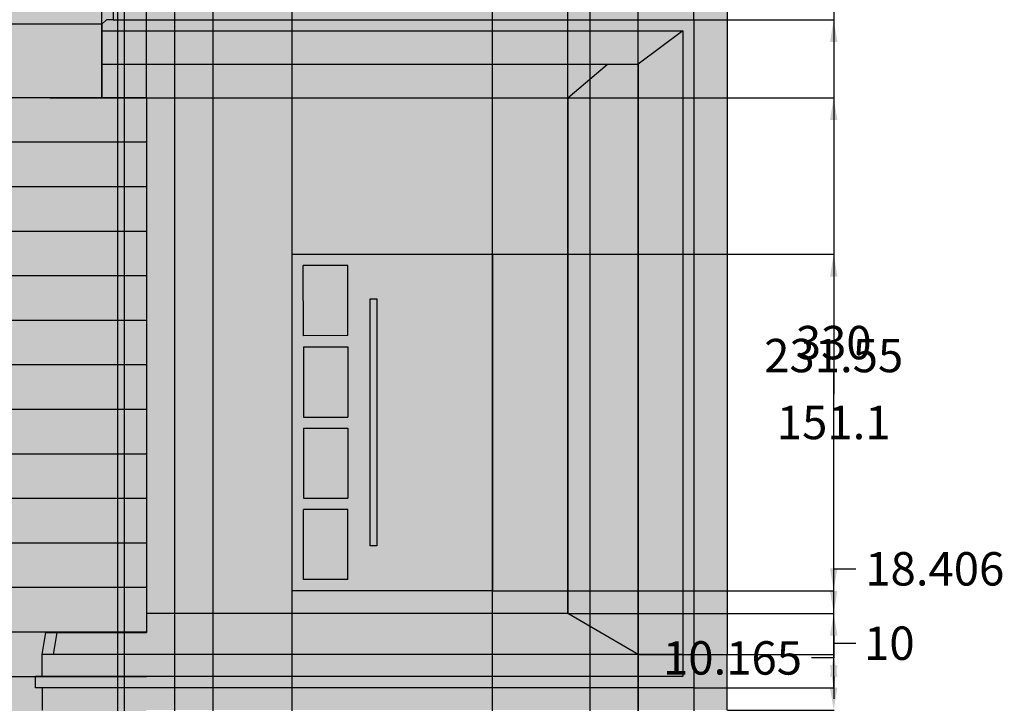
# Model space of a CAD drawing. Units: millimetres. Extents: x 131 to 845, y -20 to 1043.
# Tile 10 of 11: x 403 to 845, y 492 to 799. Entities that reach past the tile are written whole.
import ezdxf

# ---------------------------------------------------------------- set-up
doc = ezdxf.new("R2010")
doc.units = ezdxf.units.MM
doc.header["$MEASUREMENT"] = 0
for name, color, linetype, lineweight in [('A-ANNO-DIMS', 2, 'Continuous', 18), ('A-DOOR', 3, 'Continuous', 25), ('A-DOOR-PATT', 45, 'Continuous', 13), ('A-ELEV', 7, 'Continuous', 25), ('A-ELEV-PATT', 7, 'Continuous', 13), ('A-GLAZ-PATT', 143, 'Continuous', 13), ('A-WALL-PATT', 131, 'Continuous', 13)]:
    doc.layers.add(name, color=color, linetype=linetype, lineweight=lineweight)
doc.styles.get("Standard").update_dxf_attribs({"font": 'arial.ttf'})
doc.dimstyles.get("Standard").update_dxf_attribs({"dimtxt": 15, "dimasz": 10, "dimexe": 0.18, "dimexo": 0.0625, "dimgap": 5, "dimtad": 0, "dimtih": 1, "dimtoh": 1, "dimdec": 0, "dimzin": 0, "dimdsep": 46, "dimtxsty": 'Standard', "dimcen": 5, "dimadec": 0, "dimazin": 0, "dimtfac": 1, "dimtdec": 0, "dimtofl": 0, "dimtmove": 0, "dimatfit": 3, "dimfxl": 1, "dimtolj": 1, "dimtzin": 0, "dimarcsym": 0})

# ---------------------------------------------------------------- blocks, each defined once
blk = doc.blocks.new('*U5')
blk.add_line((0, 90), (0, 0))
blk = doc.blocks.new('*U6')
at = {"layer": 'A-ELEV', "color": 0, "linetype": 'ByBlock', "lineweight": -2, "transparency": 16777216, "rotation": 270}
for p in [(369.56, 763.56), (369.56, 743.56), (369.56, 723.56), (369.56, 703.56), (369.56, 683.56), (369.56, 663.56), (369.56, 643.56), (369.56, 623.56), (369.56, 603.56), (369.56, 583.56), (369.56, 563.56), (369.56, 543.56), (369.56, 523.56), (369.56, 503.56), (369.56, 483.56), (369.56, 463.56), (369.56, 443.56), (369.56, 423.56), (369.56, 403.56), (369.56, 383.56), (369.56, 363.56), (369.56, 343.56), (369.56, 323.56), (369.56, 303.56), (369.56, 283.56)]:
    blk.add_blockref('*U5', p, dxfattribs=at)
blk = doc.blocks.new('DOOR-GLASS-PANE')
for p, q in [((0, 0), (0, 31.5)), ((20, 31.5), (0, 31.5)), ((20, 0), (20, 31.5)), ((20, 0), (0, 0))]:
    blk.add_line(p, q)
blk = doc.blocks.new('*D11')
at = {"layer": 'A-ANNO-DIMS', "color": 0, "lineweight": -2, "transparency": 16777216}
for p, q in [((554.73, 464.78), (544.73, 464.78)), ((554.75, 454.78), (554.73, 464.78)), ((550.09, 454.77), (554.93, 454.78)), ((554.78, 433.28), (554.76, 444.78)), ((550.13, 423.27), (554.97, 423.28))]:
    blk.add_line(p, q, dxfattribs=at)
at = {"layer": 'A-ANNO-DIMS', "color": 0, "transparency": 16777216}
for points in [[(556.43, 444.78), (553.1, 444.77), (554.75, 454.78)], [(556.45, 433.28), (553.11, 433.27), (554.79, 423.28)]]:
    blk.add_solid(points, dxfattribs=at)
at = {"layer": 'Defpoints', "color": 0, "transparency": 16777216}
for p in [(550.02, 454.77), (554.75, 454.78), (550.07, 423.27)]:
    blk.add_point(p, dxfattribs=at)
at = {"layer": 'A-ANNO-DIMS', "color": 0, "transparency": 16777216, "insert": (399.96, 464.78), "char_height": 15, "attachment_point": 5}
blk.add_mtext('\\A1;DOOR GLASS PANE 32 TYP.', dxfattribs=at)
blk = doc.blocks.new('*D14')
at = {"layer": 'A-ANNO-DIMS', "color": 0, "lineweight": -2, "transparency": 16777216}
for p, q in [((210.52, 985.67), (162.55, 985.67)), ((162.73, 975.67), (162.73, 524.4)), ((162.73, 47.81), (162.73, 499.08)), ((459.5, 37.81), (162.55, 37.81))]:
    blk.add_line(p, q, dxfattribs=at)
at = {"layer": 'A-ANNO-DIMS', "color": 0, "transparency": 16777216}
for points in [[(161.06, 975.67), (164.4, 975.67), (162.73, 985.67)], [(161.06, 47.81), (164.4, 47.81), (162.73, 37.81)]]:
    blk.add_solid(points, dxfattribs=at)
at = {"layer": 'Defpoints', "color": 0, "transparency": 16777216}
for p in [(162.73, 985.67), (210.58, 985.67), (459.56, 37.81)]:
    blk.add_point(p, dxfattribs=at)
at = {"layer": 'A-ANNO-DIMS', "color": 0, "transparency": 16777216, "insert": (162.73, 511.74), "char_height": 15, "attachment_point": 5}
blk.add_mtext('\\A1;947.9', dxfattribs=at)
blk = doc.blocks.new('*D38')
at = {"layer": 'A-ANNO-DIMS', "color": 0, "lineweight": -2, "transparency": 16777216}
for p, q in [((439.56, 796.66), (439.56, 1033.7)), ((449.56, 1033.52), (550.85, 1033.52)), ((695.53, 1033.52), (594.24, 1033.52)), ((705.53, 798.66), (705.53, 1033.7))]:
    blk.add_line(p, q, dxfattribs=at)
at = {"layer": 'A-ANNO-DIMS', "color": 0, "transparency": 16777216}
for points in [[(449.56, 1035.18), (449.56, 1031.85), (439.56, 1033.52)], [(695.53, 1035.18), (695.53, 1031.85), (705.53, 1033.52)]]:
    blk.add_solid(points, dxfattribs=at)
at = {"layer": 'Defpoints', "color": 0, "transparency": 16777216}
for p in [(705.53, 1033.52), (439.56, 796.6), (705.53, 798.6)]:
    blk.add_point(p, dxfattribs=at)
at = {"layer": 'A-ANNO-DIMS', "color": 0, "transparency": 16777216, "insert": (572.55, 1033.52), "char_height": 15, "attachment_point": 5}
blk.add_mtext('\\A1;266', dxfattribs=at)
blk = doc.blocks.new('*D40')
at = {"layer": 'A-ANNO-DIMS', "color": 0, "lineweight": -2, "transparency": 16777216}
for p, q in [((720.6, 818.6), (768.56, 818.6)), ((768.38, 808.6), (768.38, 666.26)), ((768.38, 498.6), (768.38, 640.93)), ((720.6, 488.6), (768.56, 488.6))]:
    blk.add_line(p, q, dxfattribs=at)
at = {"layer": 'A-ANNO-DIMS', "color": 0, "transparency": 16777216}
for points in [[(766.72, 808.6), (770.05, 808.6), (768.38, 818.6)], [(766.72, 498.6), (770.05, 498.6), (768.38, 488.6)]]:
    blk.add_solid(points, dxfattribs=at)
at = {"layer": 'Defpoints', "color": 0, "transparency": 16777216}
for p in [(720.53, 818.6), (720.53, 488.6), (768.38, 488.6)]:
    blk.add_point(p, dxfattribs=at)
at = {"layer": 'A-ANNO-DIMS', "color": 0, "transparency": 16777216, "insert": (768.38, 653.6), "char_height": 15, "attachment_point": 5}
blk.add_mtext('\\A1;330', dxfattribs=at)
blk = doc.blocks.new('*D41')
at = {"layer": 'A-ANNO-DIMS', "color": 0, "lineweight": -2, "transparency": 16777216}
for p, q in [((768.38, 828.6), (768.38, 838.6)), ((768.38, 838.6), (778.38, 838.6)), ((720.6, 818.6), (768.56, 818.6)), ((705.6, 798.6), (768.56, 798.6)), ((768.38, 788.6), (768.38, 778.6))]:
    blk.add_line(p, q, dxfattribs=at)
at = {"layer": 'A-ANNO-DIMS', "color": 0, "transparency": 16777216}
for points in [[(766.72, 828.6), (770.05, 828.6), (768.38, 818.6)], [(766.72, 788.6), (770.05, 788.6), (768.38, 798.6)]]:
    blk.add_solid(points, dxfattribs=at)
at = {"layer": 'Defpoints', "color": 0, "transparency": 16777216}
for p in [(720.53, 818.6), (768.38, 818.6), (705.53, 798.6)]:
    blk.add_point(p, dxfattribs=at)
at = {"layer": 'A-ANNO-DIMS', "color": 0, "transparency": 16777216, "insert": (794.23, 838.6), "char_height": 15, "attachment_point": 5}
blk.add_mtext('\\A1;20', dxfattribs=at)
blk = doc.blocks.new('*D42')
at = {"layer": 'A-ANNO-DIMS', "color": 0, "lineweight": -2, "transparency": 16777216}
for p, q in [((459.56, 763.62), (459.56, 1033.7)), ((469.56, 1033.52), (518.83, 1033.52)), ((638.89, 1033.52), (589.63, 1033.52)), ((648.89, 763.62), (648.89, 1033.7))]:
    blk.add_line(p, q, dxfattribs=at)
at = {"layer": 'A-ANNO-DIMS', "color": 0, "transparency": 16777216}
for points in [[(469.56, 1035.18), (469.56, 1031.85), (459.56, 1033.52)], [(638.89, 1035.18), (638.89, 1031.85), (648.89, 1033.52)]]:
    blk.add_solid(points, dxfattribs=at)
at = {"layer": 'Defpoints', "color": 0, "transparency": 16777216}
for p in [(648.89, 1033.52), (459.56, 763.56), (648.89, 763.56)]:
    blk.add_point(p, dxfattribs=at)
at = {"layer": 'A-ANNO-DIMS', "color": 0, "transparency": 16777216, "insert": (554.23, 1033.52), "char_height": 15, "attachment_point": 5}
blk.add_mtext('\\A1;189.34', dxfattribs=at)
blk = doc.blocks.new('*D43')
at = {"layer": 'A-ANNO-DIMS', "color": 0, "lineweight": -2, "transparency": 16777216}
for p, q in [((648.96, 763.56), (768.56, 763.56)), ((768.38, 753.56), (768.38, 660.44)), ((768.38, 542), (768.38, 635.11)), ((648.96, 532), (768.56, 532))]:
    blk.add_line(p, q, dxfattribs=at)
at = {"layer": 'A-ANNO-DIMS', "color": 0, "transparency": 16777216}
for points in [[(766.72, 753.56), (770.05, 753.56), (768.38, 763.56)], [(766.72, 542), (770.05, 542), (768.38, 532)]]:
    blk.add_solid(points, dxfattribs=at)
at = {"layer": 'Defpoints', "color": 0, "transparency": 16777216}
for p in [(648.89, 763.56), (768.38, 763.56), (648.89, 532)]:
    blk.add_point(p, dxfattribs=at)
at = {"layer": 'A-ANNO-DIMS', "color": 0, "transparency": 16777216, "insert": (768.38, 647.78), "char_height": 15, "attachment_point": 5}
blk.add_mtext('\\A1;231.55', dxfattribs=at)
blk = doc.blocks.new('*D44')
at = {"layer": 'A-ANNO-DIMS', "color": 0, "lineweight": -2, "transparency": 16777216}
for p, q in [((429.56, 1033.52), (419.56, 1033.52)), ((439.56, 763.62), (439.56, 1033.7)), ((459.56, 763.62), (459.56, 1033.7)), ((469.56, 1033.52), (479.56, 1033.52))]:
    blk.add_line(p, q, dxfattribs=at)
at = {"layer": 'A-ANNO-DIMS', "color": 0, "transparency": 16777216}
for points in [[(429.56, 1035.18), (429.56, 1031.85), (439.56, 1033.52)], [(469.56, 1035.18), (469.56, 1031.85), (459.56, 1033.52)]]:
    blk.add_solid(points, dxfattribs=at)
at = {"layer": 'Defpoints', "color": 0, "transparency": 16777216}
for p in [(459.56, 1033.52), (439.56, 763.56), (459.56, 763.56)]:
    blk.add_point(p, dxfattribs=at)
at = {"layer": 'A-ANNO-DIMS', "color": 0, "transparency": 16777216, "insert": (495.4, 1033.52), "char_height": 15, "attachment_point": 5}
blk.add_mtext('\\A1;20', dxfattribs=at)
blk = doc.blocks.new('*D45')
at = {"layer": 'A-ANNO-DIMS', "color": 0, "lineweight": -2, "transparency": 16777216}
for p, q in [((162.73, 796.6), (162.73, 806.6)), ((162.73, 806.6), (172.73, 806.6)), ((439.5, 796.6), (162.55, 796.6)), ((162.73, 773.56), (162.73, 786.6)), ((459.5, 763.56), (162.55, 763.56))]:
    blk.add_line(p, q, dxfattribs=at)
at = {"layer": 'A-ANNO-DIMS', "color": 0, "transparency": 16777216}
for points in [[(161.06, 786.6), (164.4, 786.6), (162.73, 796.6)], [(161.06, 773.56), (164.4, 773.56), (162.73, 763.56)]]:
    blk.add_solid(points, dxfattribs=at)
at = {"layer": 'Defpoints', "color": 0, "transparency": 16777216}
for p in [(162.73, 796.6), (439.56, 796.6), (459.56, 763.56)]:
    blk.add_point(p, dxfattribs=at)
at = {"layer": 'A-ANNO-DIMS', "color": 0, "transparency": 16777216, "insert": (203, 806.6), "char_height": 15, "attachment_point": 5}
blk.add_mtext('\\A1;33.04', dxfattribs=at)
blk = doc.blocks.new('*D46')
at = {"layer": 'A-ANNO-DIMS', "color": 0, "lineweight": -2, "transparency": 16777216}
for p, q in [((648.89, 532.06), (648.89, 1033.7)), ((658.89, 1033.52), (670.53, 1033.52)), ((680.53, 513.66), (680.53, 1033.7)), ((680.53, 1033.52), (690.53, 1033.52))]:
    blk.add_line(p, q, dxfattribs=at)
at = {"layer": 'A-ANNO-DIMS', "color": 0, "transparency": 16777216}
for points in [[(658.89, 1035.18), (658.89, 1031.85), (648.89, 1033.52)], [(670.53, 1035.18), (670.53, 1031.85), (680.53, 1033.52)]]:
    blk.add_solid(points, dxfattribs=at)
at = {"layer": 'Defpoints', "color": 0, "transparency": 16777216}
for p in [(680.53, 1033.52), (648.89, 532), (680.53, 513.6)]:
    blk.add_point(p, dxfattribs=at)
at = {"layer": 'A-ANNO-DIMS', "color": 0, "transparency": 16777216, "insert": (720.81, 1033.52), "char_height": 15, "attachment_point": 5}
blk.add_mtext('\\A1;31.64', dxfattribs=at)
blk = doc.blocks.new('*D47')
at = {"layer": 'A-ANNO-DIMS', "color": 0, "lineweight": -2, "transparency": 16777216}
for p, q in [((768.38, 542), (768.38, 552)), ((768.38, 552), (778.38, 552)), ((648.96, 532), (768.56, 532)), ((680.6, 513.6), (768.56, 513.6)), ((768.38, 503.6), (768.38, 493.6))]:
    blk.add_line(p, q, dxfattribs=at)
at = {"layer": 'A-ANNO-DIMS', "color": 0, "transparency": 16777216}
for points in [[(766.72, 542), (770.05, 542), (768.38, 532)], [(766.72, 503.6), (770.05, 503.6), (768.38, 513.6)]]:
    blk.add_solid(points, dxfattribs=at)
at = {"layer": 'Defpoints', "color": 0, "transparency": 16777216}
for p in [(648.89, 532), (768.38, 532), (680.53, 513.6)]:
    blk.add_point(p, dxfattribs=at)
at = {"layer": 'A-ANNO-DIMS', "color": 0, "transparency": 16777216, "insert": (813.81, 552), "char_height": 15, "attachment_point": 5}
blk.add_mtext('\\A1;18.406', dxfattribs=at)
blk = doc.blocks.new('*D48')
at = {"layer": 'A-ANNO-DIMS', "color": 0, "lineweight": -2, "transparency": 16777216}
for p, q in [((680.53, 513.53), (680.53, -10.22)), ((705.53, 498.53), (705.53, -10.22)), ((670.53, -10.04), (660.53, -10.04)), ((715.53, -10.04), (725.53, -10.04))]:
    blk.add_line(p, q, dxfattribs=at)
at = {"layer": 'A-ANNO-DIMS', "color": 0, "transparency": 16777216}
for points in [[(670.53, -8.37), (670.53, -11.7), (680.53, -10.04)], [(715.53, -8.37), (715.53, -11.7), (705.53, -10.04)]]:
    blk.add_solid(points, dxfattribs=at)
at = {"layer": 'Defpoints', "color": 0, "transparency": 16777216}
for p in [(680.53, 513.6), (705.53, 498.6), (705.53, -10.04)]:
    blk.add_point(p, dxfattribs=at)
at = {"layer": 'A-ANNO-DIMS', "color": 0, "transparency": 16777216, "insert": (741.46, -10.04), "char_height": 15, "attachment_point": 5}
blk.add_mtext('\\A1;25', dxfattribs=at)
blk = doc.blocks.new('*D49')
at = {"layer": 'A-ANNO-DIMS', "color": 0, "lineweight": -2, "transparency": 16777216}
for p, q in [((768.38, 508.6), (768.38, 518.6)), ((768.38, 518.6), (778.38, 518.6)), ((705.6, 498.6), (768.56, 498.6)), ((720.6, 488.6), (768.56, 488.6)), ((768.38, 478.6), (768.38, 468.6))]:
    blk.add_line(p, q, dxfattribs=at)
at = {"layer": 'A-ANNO-DIMS', "color": 0, "transparency": 16777216}
for points in [[(766.72, 508.6), (770.05, 508.6), (768.38, 498.6)], [(766.72, 478.6), (770.05, 478.6), (768.38, 488.6)]]:
    blk.add_solid(points, dxfattribs=at)
at = {"layer": 'Defpoints', "color": 0, "transparency": 16777216}
for p in [(705.53, 498.6), (768.38, 498.6), (720.53, 488.6)]:
    blk.add_point(p, dxfattribs=at)
at = {"layer": 'A-ANNO-DIMS', "color": 0, "transparency": 16777216, "insert": (793.4, 518.6), "char_height": 15, "attachment_point": 5}
blk.add_mtext('\\A1;10', dxfattribs=at)
blk = doc.blocks.new('*D54')
at = {"layer": 'A-ANNO-DIMS', "color": 0, "lineweight": -2, "transparency": 16777216}
for p, q in [((525.05, 693.33), (525.05, 1033.7)), ((535.05, 1033.52), (554.33, 1033.52)), ((605.05, 1033.52), (585.76, 1033.52)), ((615.05, 693.33), (615.05, 1033.7))]:
    blk.add_line(p, q, dxfattribs=at)
at = {"layer": 'A-ANNO-DIMS', "color": 0, "transparency": 16777216}
for points in [[(535.05, 1035.18), (535.05, 1031.85), (525.05, 1033.52)], [(605.05, 1035.18), (605.05, 1031.85), (615.05, 1033.52)]]:
    blk.add_solid(points, dxfattribs=at)
at = {"layer": 'Defpoints', "color": 0, "transparency": 16777216}
for p in [(615.05, 1033.52), (525.05, 693.27), (615.05, 693.27)]:
    blk.add_point(p, dxfattribs=at)
at = {"layer": 'A-ANNO-DIMS', "color": 0, "transparency": 16777216, "insert": (570.05, 1033.52), "char_height": 15, "attachment_point": 5}
blk.add_mtext('\\A1;90', dxfattribs=at)
blk = doc.blocks.new('*D55')
at = {"layer": 'A-ANNO-DIMS', "color": 0, "lineweight": -2, "transparency": 16777216}
for p, q in [((615.11, 693.27), (768.56, 693.27)), ((768.38, 683.27), (768.38, 630.38)), ((768.38, 552.17), (768.38, 605.06)), ((615.11, 542.17), (768.56, 542.17))]:
    blk.add_line(p, q, dxfattribs=at)
at = {"layer": 'A-ANNO-DIMS', "color": 0, "transparency": 16777216}
for points in [[(766.72, 683.27), (770.05, 683.27), (768.38, 693.27)], [(766.72, 552.17), (770.05, 552.17), (768.38, 542.17)]]:
    blk.add_solid(points, dxfattribs=at)
at = {"layer": 'Defpoints', "color": 0, "transparency": 16777216}
for p in [(615.05, 693.27), (768.38, 693.27), (615.05, 542.17)]:
    blk.add_point(p, dxfattribs=at)
at = {"layer": 'A-ANNO-DIMS', "color": 0, "transparency": 16777216, "insert": (768.38, 617.72), "char_height": 15, "attachment_point": 5}
blk.add_mtext('\\A1;151.1', dxfattribs=at)
blk = doc.blocks.new('*D56')
at = {"layer": 'A-ANNO-DIMS', "color": 0, "lineweight": -2, "transparency": 16777216}
for p, q in [((449.56, 1033.52), (439.56, 1033.52)), ((459.56, 763.62), (459.56, 1033.7)), ((525.05, 693.33), (525.05, 1033.7)), ((535.05, 1033.52), (545.05, 1033.52))]:
    blk.add_line(p, q, dxfattribs=at)
at = {"layer": 'A-ANNO-DIMS', "color": 0, "transparency": 16777216}
for points in [[(449.56, 1035.18), (449.56, 1031.85), (459.56, 1033.52)], [(535.05, 1035.18), (535.05, 1031.85), (525.05, 1033.52)]]:
    blk.add_solid(points, dxfattribs=at)
at = {"layer": 'Defpoints', "color": 0, "transparency": 16777216}
for p in [(525.05, 1033.52), (459.56, 763.56), (525.05, 693.27)]:
    blk.add_point(p, dxfattribs=at)
at = {"layer": 'A-ANNO-DIMS', "color": 0, "transparency": 16777216, "insert": (492.3, 1033.52), "char_height": 15, "attachment_point": 5}
blk.add_mtext('\\A1;65.49', dxfattribs=at)
blk = doc.blocks.new('*D57')
at = {"layer": 'A-ANNO-DIMS', "color": 0, "lineweight": -2, "transparency": 16777216}
for p, q in [((768.38, 552.17), (768.38, 562.17)), ((615.11, 542.17), (768.56, 542.17)), ((648.96, 532), (768.56, 532)), ((768.38, 522), (768.38, 512)), ((768.38, 512), (758.38, 512))]:
    blk.add_line(p, q, dxfattribs=at)
at = {"layer": 'A-ANNO-DIMS', "color": 0, "transparency": 16777216}
for points in [[(766.72, 552.17), (770.05, 552.17), (768.38, 542.17)], [(766.72, 522), (770.05, 522), (768.38, 532)]]:
    blk.add_solid(points, dxfattribs=at)
at = {"layer": 'Defpoints', "color": 0, "transparency": 16777216}
for p in [(615.05, 542.17), (648.89, 532), (768.38, 532)]:
    blk.add_point(p, dxfattribs=at)
at = {"layer": 'A-ANNO-DIMS', "color": 0, "transparency": 16777216, "insert": (722.9, 512), "char_height": 15, "attachment_point": 5}
blk.add_mtext('\\A1;10.165', dxfattribs=at)
blk = doc.blocks.new('*D58')
at = {"layer": 'A-ANNO-DIMS', "color": 0, "lineweight": -2, "transparency": 16777216}
for p, q in [((525.05, 459.87), (525.05, 1033.7)), ((535.05, 1033.52), (554.33, 1033.52)), ((605.05, 1033.52), (585.76, 1033.52)), ((615.05, 459.87), (615.05, 1033.7))]:
    blk.add_line(p, q, dxfattribs=at)
at = {"layer": 'A-ANNO-DIMS', "color": 0, "transparency": 16777216}
for points in [[(535.05, 1035.18), (535.05, 1031.85), (525.05, 1033.52)], [(605.05, 1035.18), (605.05, 1031.85), (615.05, 1033.52)]]:
    blk.add_solid(points, dxfattribs=at)
at = {"layer": 'Defpoints', "color": 0, "transparency": 16777216}
for p in [(615.05, 1033.52), (525.05, 459.8), (615.05, 459.8)]:
    blk.add_point(p, dxfattribs=at)
at = {"layer": 'A-ANNO-DIMS', "color": 0, "transparency": 16777216, "insert": (570.05, 1033.52), "char_height": 15, "attachment_point": 5}
blk.add_mtext('\\A1;90', dxfattribs=at)
blk = doc.blocks.new('*D75')
at = {"layer": 'A-ANNO-DIMS', "color": 0, "lineweight": -2, "transparency": 16777216}
for p, q in [((462.24, 1033.52), (452.24, 1033.52)), ((472.24, 310.22), (472.24, 1033.7)), ((489.56, 300.22), (489.56, 1033.7)), ((499.56, 1033.52), (509.56, 1033.52))]:
    blk.add_line(p, q, dxfattribs=at)
at = {"layer": 'A-ANNO-DIMS', "color": 0, "transparency": 16777216}
for points in [[(462.24, 1035.18), (462.24, 1031.85), (472.24, 1033.52)], [(499.56, 1035.18), (499.56, 1031.85), (489.56, 1033.52)]]:
    blk.add_solid(points, dxfattribs=at)
at = {"layer": 'Defpoints', "color": 0, "transparency": 16777216}
for p in [(489.56, 1033.52), (472.24, 310.16), (489.56, 300.16)]:
    blk.add_point(p, dxfattribs=at)
at = {"layer": 'A-ANNO-DIMS', "color": 0, "transparency": 16777216, "insert": (539.08, 1033.52), "char_height": 15, "attachment_point": 5}
blk.add_mtext('\\A1;17.32', dxfattribs=at)
blk = doc.blocks.new('*D77')
at = {"layer": 'A-ANNO-DIMS', "color": 0, "lineweight": -2, "transparency": 16777216}
for p, q in [((648.88, 1033.52), (638.88, 1033.52)), ((658.88, 312.72), (658.88, 1033.7)), ((680.53, 300.22), (680.53, 1033.7)), ((690.53, 1033.52), (700.53, 1033.52))]:
    blk.add_line(p, q, dxfattribs=at)
at = {"layer": 'A-ANNO-DIMS', "color": 0, "transparency": 16777216}
for points in [[(648.88, 1035.18), (648.88, 1031.85), (658.88, 1033.52)], [(690.53, 1035.18), (690.53, 1031.85), (680.53, 1033.52)]]:
    blk.add_solid(points, dxfattribs=at)
at = {"layer": 'Defpoints', "color": 0, "transparency": 16777216}
for p in [(680.53, 1033.52), (658.88, 312.66), (680.53, 300.16)]:
    blk.add_point(p, dxfattribs=at)
at = {"layer": 'A-ANNO-DIMS', "color": 0, "transparency": 16777216, "insert": (731.03, 1033.52), "char_height": 15, "attachment_point": 5}
blk.add_mtext('\\A1;21.65', dxfattribs=at)
blk = doc.blocks.new('*D99')
at = {"layer": 'A-ANNO-DIMS', "color": 0, "lineweight": -2, "transparency": 16777216}
for p, q in [((449.56, 833.53), (449.56, -10.22)), ((446.56, 818.53), (446.56, -10.22)), ((436.56, -10.04), (426.56, -10.04)), ((459.56, -10.04), (469.56, -10.04))]:
    blk.add_line(p, q, dxfattribs=at)
at = {"layer": 'A-ANNO-DIMS', "color": 0, "transparency": 16777216}
for points in [[(436.56, -8.37), (436.56, -11.7), (446.56, -10.04)], [(459.56, -8.37), (459.56, -11.7), (449.56, -10.04)]]:
    blk.add_solid(points, dxfattribs=at)
at = {"layer": 'Defpoints', "color": 0, "transparency": 16777216}
for p in [(449.56, 833.6), (446.56, 818.6), (449.56, -10.04)]:
    blk.add_point(p, dxfattribs=at)
at = {"layer": 'A-ANNO-DIMS', "color": 0, "transparency": 16777216, "insert": (479.47, -10.04), "char_height": 15, "attachment_point": 5}
blk.add_mtext('\\A1;3', dxfattribs=at)

msp = doc.modelspace()

# ---------------------------------------------------------------- hatches: boundary and pattern name
at = {"layer": 'A-DOOR-PATT'}
h = msp.add_hatch(color=256, dxfattribs=at)
h.dxf.hatch_style = 1
h.paths.add_polyline_path([(615.0467, 459.8046), (525.0467, 459.8046), (525.0467, 323.1596), (530.0467, 323.1596), (530.0467, 345.2044), (550.0467, 345.2044), (550.0467, 323.1596), (570.0467, 323.1596), (570.0467, 305.1596), (570.0467, 303.6234), (572.0453, 303.6234), (572.0467, 305.1596), (572.0467, 323.1596), (615.0467, 323.1596)])
h.paths.add_polyline_path([(563.0467, 328.8046), (560.0467, 328.8046), (560.0467, 439.8046), (563.0467, 439.8046)], flags=16)
h.paths.add_polyline_path([(550.0467, 386.7044), (530.0467, 386.7044), (530.0467, 418.2044), (550.0467, 418.2044)], flags=16)
h.paths.add_polyline_path([(550.0467, 381.7044), (550.0467, 350.2044), (530.0467, 350.2044), (530.0467, 381.7044)], flags=16)
h.paths.add_polyline_path([(550.0467, 423.2044), (530.0467, 423.2044), (530.0467, 454.8046), (550.0467, 454.8046)], flags=16)
h.paths.add_polyline_path([(615.0467, 693.2667), (525.0467, 693.2667), (525.0467, 542.1664), (615.0467, 542.1664)])
h.paths.add_polyline_path([(563.0467, 562.2667), (560.0467, 562.2667), (560.0467, 673.2667), (563.0467, 673.2667)], flags=16)
h.paths.add_polyline_path([(550.0467, 583.6664), (530.0467, 583.6664), (530.0467, 615.1664), (550.0467, 615.1664)], flags=16)
h.paths.add_polyline_path([(550.0467, 578.6664), (550.0467, 547.1664), (530.0467, 547.1664), (530.0467, 578.6664)], flags=16)
h.paths.add_polyline_path([(550.0467, 620.1664), (530.0467, 620.1664), (530.0467, 651.6664), (550.0467, 651.6664)], flags=16)
h.paths.add_polyline_path([(550.0467, 656.6664), (530.0467, 656.6664), (530.0467, 688.2667), (550.0467, 688.2667)], flags=16)
at = {"layer": 'A-ELEV-PATT'}
h = msp.add_hatch(color=256, dxfattribs=at)
h.set_gradient(color1=(255, 255, 255), color2=(147, 149, 152), name='INVSPHERICAL')
h.paths.add_polyline_path([(705.5349, 798.5953), (444.5586, 798.5953), (441.5586, 798.5953), (439.5586, 796.5953), (439.5586, 793.5953), (444.5586, 793.5953), (700.5349, 793.5953), (700.5349, 513.5953), (700.5349, 503.5953), (680.5349, 503.5953), (680.5349, 498.5953), (705.5349, 498.5953), (705.5349, 513.5953)])
h.paths.add_polyline_path([(680.5349, 503.5953), (409.6606, 503.5953), (409.6606, 498.5953), (680.5349, 498.5953)])
h = msp.add_hatch(color=256, dxfattribs=at)
h.set_gradient(color1=(255, 255, 255), color2=(99, 100, 102), name='INVCYLINDER')
h.paths.add_polyline_path([(705.5349, 798.5953), (444.5586, 798.5953), (441.5586, 798.5953), (439.5586, 796.5953), (439.5586, 793.5953), (444.5586, 793.5953), (700.5349, 793.5953), (700.5349, 513.5953), (700.5349, 503.5953), (680.5349, 503.5953), (680.5349, 498.5953), (705.5349, 498.5953), (705.5349, 513.5953)])
at = {"layer": 'A-ELEV-PATT', "transparency": 33554681}
h = msp.add_hatch(color=256, dxfattribs=at)
h.set_gradient(color1=(147, 149, 152), color2=(192, 192, 192), name='CYLINDER')
h.paths.add_polyline_path([(369.5586, 763.5561), (369.5586, 743.5561), (459.5586, 743.5561), (459.5586, 763.5561)])
h.paths.add_polyline_path([(459.5586, 703.5561), (459.5586, 723.5561), (369.5586, 723.5561), (369.5586, 703.5561)])
h.paths.add_polyline_path([(459.5586, 663.5561), (459.5586, 683.5561), (369.5586, 683.5561), (369.5586, 663.5561)])
h.paths.add_polyline_path([(459.5586, 623.5561), (459.5586, 643.5561), (369.5586, 643.5561), (369.5586, 623.5561)])
h.paths.add_polyline_path([(459.5586, 583.5561), (459.5586, 603.5561), (369.5586, 603.5561), (369.5586, 583.5561)])
h.paths.add_polyline_path([(459.5586, 543.5561), (459.5586, 563.5561), (369.5586, 563.5561), (369.5586, 543.5561)])
h.paths.add_polyline_path([(369.5586, 523.5561), (369.5586, 503.5561), (409.6606, 503.5561), (409.6606, 503.5953), (412.6606, 503.5953), (412.6606, 513.5953), (414.417, 523.5561)])
h.paths.add_polyline_path([(369.5586, 483.5561), (369.5586, 463.5561), (459.5586, 463.5561), (459.5586, 483.5561)])
h.paths.add_polyline_path([(459.5586, 423.5561), (459.5586, 443.5561), (369.5586, 443.5561), (369.5586, 423.5561)])
h.paths.add_polyline_path([(369.5586, 403.5561), (369.5586, 383.5561), (459.5586, 383.5561), (459.5586, 403.5561)])
h.paths.add_polyline_path([(459.5586, 343.5561), (459.5586, 363.5561), (369.5586, 363.5561), (369.5586, 343.5561)])
h.paths.add_polyline_path([(369.5586, 323.5561), (369.5586, 303.5561), (459.5586, 303.5561), (459.5586, 323.5561)])
h = msp.add_hatch(color=256, dxfattribs=at)
h.set_gradient(color1=(255, 255, 255), color2=(199, 200, 202), name='INVSPHERICAL')
h.paths.add_polyline_path([(459.5586, 532.0012), (648.8943, 532.0012), (648.8943, 763.5561), (459.5586, 763.5561)])
h.paths.add_polyline_path([(525.0467, 693.2667), (615.0467, 693.2667), (615.0467, 542.1664), (525.0467, 542.1664)], flags=16)
h.paths.add_polyline_path([(530.0467, 688.2667), (550.0467, 688.2667), (550.0467, 656.6664), (530.0467, 656.6664)], flags=0)
h.paths.add_polyline_path([(530.0467, 651.6664), (550.0467, 651.6664), (550.0467, 620.1664), (530.0467, 620.1664)], flags=0)
h.paths.add_polyline_path([(560.0467, 673.2667), (563.0467, 673.2667), (563.0467, 562.2667), (560.0467, 562.2667)], flags=0)
h.paths.add_polyline_path([(530.0467, 615.1664), (550.0467, 615.1664), (550.0467, 583.6664), (530.0467, 583.6664)], flags=0)
h.paths.add_polyline_path([(530.0467, 578.6664), (550.0467, 578.6664), (550.0467, 547.1664), (530.0467, 547.1664)], flags=0)
h = msp.add_hatch(color=256, dxfattribs=at)
h.set_gradient(color1=(147, 149, 152), color2=(192, 192, 192), name='CURVED')
h.paths.add_polyline_path([(369.5586, 743.5561), (369.5586, 723.5561), (459.5586, 723.5561), (459.5586, 743.5561)])
h.paths.add_polyline_path([(369.5586, 703.5561), (369.5586, 683.5561), (459.5586, 683.5561), (459.5586, 703.5561)])
h.paths.add_polyline_path([(459.5586, 643.5561), (459.5586, 663.5561), (369.5586, 663.5561), (369.5586, 643.5561)])
h.paths.add_polyline_path([(459.5586, 603.5561), (459.5586, 623.5561), (369.5586, 623.5561), (369.5586, 603.5561)])
h.paths.add_polyline_path([(369.5586, 583.5561), (369.5586, 563.5561), (459.5586, 563.5561), (459.5586, 583.5561)])
h.paths.add_polyline_path([(369.5586, 543.5561), (369.5586, 523.5561), (459.5586, 523.5561), (459.5586, 543.5561)])
h.paths.add_polyline_path([(459.5586, 483.5561), (459.5586, 488.5953), (412.6606, 488.5953), (412.6606, 498.5953), (409.6606, 498.5953), (409.6606, 503.5561), (369.5586, 503.5561), (369.5586, 483.5561)])
h.paths.add_polyline_path([(369.5586, 463.5561), (369.5586, 443.5561), (459.5586, 443.5561), (459.5586, 463.5561)])
h.paths.add_polyline_path([(369.5586, 423.5561), (369.5586, 403.5561), (459.5586, 403.5561), (459.5586, 423.5561)])
h.paths.add_polyline_path([(369.5586, 383.5561), (369.5586, 363.5561), (459.5586, 363.5561), (459.5586, 383.5561)])
h.paths.add_polyline_path([(369.5586, 343.5561), (369.5586, 323.5561), (459.5586, 323.5561), (459.5586, 343.5561)])
h.paths.add_polyline_path([(369.5586, 303.5561), (369.5586, 283.5561), (459.5586, 283.5561), (459.5586, 303.5561)])
h = msp.add_hatch(color=256, dxfattribs=at)
h.set_gradient(color1=(79, 2, 22), color2=(98, 46, 19), name='SPHERICAL')
h.paths.add_polyline_path([(615.0467, 693.2667), (525.0467, 693.2667), (525.0467, 542.1664), (615.0467, 542.1664)])
h.paths.add_polyline_path([(563.0467, 562.2667), (560.0467, 562.2667), (560.0467, 673.2667), (563.0467, 673.2667)], flags=16)
h.paths.add_polyline_path([(550.0467, 620.1664), (530.0467, 620.1664), (530.0467, 651.6664), (550.0467, 651.6664)], flags=16)
h.paths.add_polyline_path([(550.0467, 615.1664), (550.0467, 583.6664), (530.0467, 583.6664), (530.0467, 615.1664)], flags=16)
h.paths.add_polyline_path([(550.0467, 656.6664), (530.0467, 656.6664), (530.0467, 688.2667), (550.0467, 688.2667)], flags=16)
h.paths.add_polyline_path([(550.0467, 578.6664), (550.0467, 547.1664), (530.0467, 547.1664), (530.0467, 578.6664)], flags=16)
h = msp.add_hatch(color=256, dxfattribs=at)
h.set_gradient(color1=(99, 100, 102), color2=(199, 200, 202), name='SPHERICAL')
h.paths.add_polyline_path([(550.0467, 688.2667), (530.0467, 688.2667), (530.0467, 656.6664), (550.0467, 656.6664)])
h.paths.add_polyline_path([(530.0467, 620.1664), (550.0467, 620.1664), (550.0467, 651.6664), (530.0467, 651.6664)])
h.paths.add_polyline_path([(550.0467, 615.1664), (530.0467, 615.1664), (530.0467, 583.6664), (550.0467, 583.6664)])
h.paths.add_polyline_path([(550.0467, 547.1664), (550.0467, 578.6664), (530.0467, 578.6664), (530.0467, 547.1664)])
h.paths.add_polyline_path([(563.0467, 673.2667), (560.0467, 673.2667), (560.0467, 562.2667), (563.0467, 562.2667)])
h.paths.add_polyline_path([(550.0467, 423.2044), (550.0467, 454.8046), (530.0467, 454.8046), (530.0467, 423.2044)])
h.paths.add_polyline_path([(550.0467, 418.2044), (530.0467, 418.2044), (530.0467, 386.7044), (550.0467, 386.7044)])
h.paths.add_polyline_path([(530.0467, 350.2044), (550.0467, 350.2044), (550.0467, 381.7044), (530.0467, 381.7044)])
h.paths.add_polyline_path([(550.0467, 323.1596), (550.0467, 345.2044), (530.0467, 345.2044), (530.0467, 323.1596)])
h.paths.add_polyline_path([(563.0467, 439.8046), (560.0467, 439.8046), (560.0467, 328.8046), (563.0467, 328.8046)])
at = {"layer": 'A-ELEV-PATT'}
h = msp.add_hatch(color=256, dxfattribs=at)
h.set_gradient(color1=(255, 255, 255), color2=(247, 171, 174), name='INVSPHERICAL')
h.paths.add_polyline_path([(412.6606, 513.5953), (417.7378, 513.5953), (419.4742, 523.4433), (414.3971, 523.4433)])
h = msp.add_hatch(color=256, dxfattribs=at)
h.set_gradient(color1=(255, 255, 255), color2=(147, 149, 152), name='CURVED')
h.paths.add_polyline_path([(412.6606, 513.5953), (412.6606, 503.5953), (700.5349, 503.5953), (700.5349, 513.5953)])
at = {"layer": 'A-GLAZ-PATT'}
h = msp.add_hatch(color=256, dxfattribs=at)
h.dxf.hatch_style = 1
h.paths.add_polyline_path([(680.5349, 778.6714), (666.7118, 778.6714), (648.8943, 763.5561), (648.8943, 532.0012), (680.5349, 513.5953)])
h.paths.add_polyline_path([(666.7118, 778.6714), (439.5586, 778.6714), (439.5586, 763.5561), (459.5586, 763.5561), (648.8943, 763.5561)])
h.paths.add_polyline_path([(700.5349, 793.5953), (444.5586, 793.5953), (439.5586, 793.5953), (439.5586, 778.6714), (666.7118, 778.6714), (680.5349, 778.6714)])
h.paths.add_polyline_path([(700.5349, 793.5953), (680.5349, 778.6714), (680.5349, 513.5953), (700.5349, 513.5953)])
h.paths.add_polyline_path([(648.8943, 532.0012), (570.0467, 532.0012), (570.0467, 513.5953), (680.5349, 513.5953)])
h.paths.add_polyline_path([(570.0467, 532.0012), (459.5586, 532.0012), (459.5586, 523.4433), (419.4742, 523.4433), (417.7378, 513.5953), (570.0467, 513.5953)])
at = {"layer": 'A-WALL-PATT'}
h = msp.add_hatch(color=256, dxfattribs=at)
h.dxf.hatch_style = 1
h.paths.add_polyline_path([(449.5586, 833.5953), (451.6297, 835.6663), (451.6297, 885.6663), (466.6297, 885.6663), (466.6297, 891.3345), (330.6595, 891.3345), (330.6595, 856.8345), (292.1595, 856.8345), (292.1595, 798.4332), (336.1595, 798.4332), (336.1595, 178.4332), (246.1595, 178.4332), (246.1595, 798.4332), (290.1595, 798.4332), (290.1595, 856.8345), (259.6595, 856.8345), (255.6595, 860.8345), (255.6595, 927.8345), (290.1595, 927.8345), (290.1595, 960.6663), (216.2327, 960.6663), (216.2327, 60.3131), (459.5586, 60.3131), (459.5586, 97.8131), (459.5586, 252.07), (459.5586, 283.5561), (369.5586, 283.5561), (369.5586, 763.5561), (439.5586, 763.5561), (439.5586, 778.6714), (439.5586, 793.5953), (439.5586, 796.5953), (441.5586, 798.5953), (444.5586, 798.5953), (444.5586, 813.5953), (444.5586, 816.5953), (446.5586, 818.5953), (449.5586, 818.5953)])
h.paths.add_polyline_path([(466.6297, 960.6663), (292.1595, 960.6663), (292.1595, 927.8345), (326.6595, 927.8345), (330.6595, 923.8345), (330.6595, 893.3345), (466.6297, 893.3345)], flags=17)
h.paths.add_polyline_path([(720.5349, 813.5953), (720.5349, 818.5953), (710.5349, 818.5953), (449.5586, 818.5953), (446.5586, 818.5953), (444.5586, 816.5953), (444.5586, 813.5953), (444.5586, 798.5953), (705.5349, 798.5953), (705.5349, 513.5953), (705.5349, 498.5953), (680.5349, 498.5953), (680.5349, 488.5953), (705.5349, 488.5953), (720.5349, 488.5953), (720.5349, 513.5953)])
h.paths.add_polyline_path([(680.5349, 498.5953), (412.6606, 498.5953), (412.6606, 488.5953), (680.5349, 488.5953)])

# ---------------------------------------------------------------- linework, layer by layer
at = {"layer": 'A-DOOR'}
for p, q in [((525.0467, 693.2667), (615.0467, 693.2667)), ((525.0467, 542.1664), (525.0467, 693.2667)), ((615.0467, 693.2667), (615.0467, 542.1664)), ((560.0467, 656.6664), (560.0467, 673.2667)), ((615.0467, 542.1664), (525.0467, 542.1664))]:
    msp.add_line(p, q, dxfattribs=at)
msp.add_lwpolyline([(560.0467, 673.2667), (563.0467, 673.2667), (563.0467, 562.2667), (560.0467, 562.2667)], close=True, dxfattribs=at)
at = {"layer": 'A-ELEV'}
for p, q in [((444.5586, 813.5953), (444.5586, 798.5953)), ((720.5349, 813.5953), (720.5349, 513.5953)), ((441.5586, 798.5953), (439.5586, 796.5953)), ((439.5586, 796.5953), (439.5586, 793.5953)), ((444.5586, 798.5953), (441.5586, 798.5953)), ((444.5586, 798.5953), (705.5349, 798.5953)), ((705.5349, 798.5953), (705.5349, 513.5953)), ((439.5586, 793.5953), (444.5586, 793.5953)), ((439.5586, 793.5953), (439.5586, 778.6714)), ((444.5586, 793.5953), (700.5349, 793.5953)), ((700.5349, 793.5953), (680.5349, 778.6714)), ((700.5349, 793.5953), (700.5349, 513.5953)), ((439.5586, 778.6714), (680.5349, 778.6714)), ((439.5586, 778.6714), (439.5586, 763.5561)), ((648.8943, 763.5561), (666.7118, 778.6714)), ((680.5349, 778.6714), (680.5349, 513.5953)), ((416.1749, 763.5561), (648.8943, 763.5561)), ((439.5586, 763.5561), (459.5586, 763.5561)), ((459.5586, 763.5561), (459.5586, 523.4433)), ((648.8943, 763.5561), (648.8943, 532.0012)), ((648.8943, 532.0012), (459.5586, 532.0012)), ((680.5349, 513.5953), (648.8943, 532.0012)), ((412.6606, 513.5953), (414.3971, 523.4433)), ((414.3971, 523.4433), (459.5586, 523.4433)), ((417.7378, 513.5953), (419.4742, 523.4433)), ((700.5349, 513.5953), (412.6606, 513.5953)), ((412.6606, 503.5953), (412.6606, 513.5953)), ((700.5349, 513.5953), (700.5349, 503.5953)), ((705.5349, 513.5953), (705.5349, 498.5953)), ((720.5349, 488.5953), (720.5349, 513.5953)), ((700.5349, 503.5953), (409.6606, 503.5953)), ((409.6606, 498.5953), (409.6606, 503.5953)), ((705.5349, 498.5953), (409.6606, 498.5953)), ((412.6606, 498.5953), (412.6606, 488.5953)), ((680.5349, 498.5953), (680.5349, 488.5953))]:
    msp.add_line(p, q, dxfattribs=at)

# ---------------------------------------------------------------- block references
at = {"layer": 'A-DOOR'}
for p, rotation in [((530.0696, 656.7018), 0.0823557908083867), ((550.0465, 651.6667), 180), ((550.0465, 615.1667), 180)]:
    msp.add_blockref('DOOR-GLASS-PANE', p, dxfattribs=dict(at, rotation=rotation))
msp.add_blockref('DOOR-GLASS-PANE', (530.047, 547.166), dxfattribs=at)
at = {"layer": 'A-ELEV'}
msp.add_blockref('*U6', (0, 0), dxfattribs=at)

# ---------------------------------------------------------------- dimensions: what is measured, and where the dimension line sits
at = {"layer": 'A-ANNO-DIMS'}
for base, p1, p2, override, picture, middle in [((459.5586, 1033.5163), (439.5586, 763.5561), (459.5586, 763.5561), {"dimdec": 0, "dimlfac": 1, "dimrnd": 0, "dimzin": 0, "dimdsep": 46, "dimlunit": 2}, '*D44', (495.4044, 1033.5163)), ((705.5349, 1033.5163), (439.5586, 796.5953), (705.5349, 798.5953), {"dimdec": 0, "dimlfac": 1, "dimrnd": 0, "dimzin": 0, "dimdsep": 46, "dimlunit": 2}, '*D38', (572.5467, 1033.5163)), ((525.0467, 1033.5163), (459.5586, 763.5561), (525.0467, 693.2667), {"dimdec": 2, "dimlfac": 1, "dimrnd": 0, "dimzin": 0, "dimdsep": 46, "dimlunit": 2}, '*D56', (492.3027, 1033.5163)), ((489.5586, 1033.5163), (472.2381, 310.1596), (489.5586, 300.1596), {"dimdec": 2, "dimlfac": 1, "dimrnd": 0, "dimzin": 0, "dimdsep": 46, "dimlunit": 2}, '*D75', (539.0845, 1033.5163)), ((648.8943, 1033.5163), (459.5586, 763.5561), (648.8943, 763.5561), {"dimdec": 2, "dimlfac": 1, "dimrnd": 0, "dimzin": 0, "dimdsep": 46, "dimlunit": 2}, '*D42', (554.2265, 1033.5163)), ((615.0467, 1033.5163), (525.0467, 693.2667), (615.0467, 693.2667), {"dimdec": 0, "dimlfac": 1, "dimrnd": 0, "dimzin": 0, "dimdsep": 46, "dimlunit": 2}, '*D54', (570.0467, 1033.5163)), ((615.0467, 1033.5163), (525.0467, 459.8046), (615.0467, 459.8046), {"dimdec": 0, "dimlfac": 1, "dimrnd": 0, "dimzin": 0, "dimdsep": 46, "dimlunit": 2}, '*D58', (570.0467, 1033.5163)), ((680.5349, 1033.5163), (658.8842, 312.6596), (680.5349, 300.1596), {"dimdec": 2, "dimlfac": 1, "dimrnd": 0, "dimzin": 0, "dimdsep": 46, "dimlunit": 2}, '*D77', (731.0277, 1033.5163)), ((680.5349, 1033.5163), (648.8943, 532.0012), (680.5349, 513.5953), {"dimdec": 2, "dimlfac": 1, "dimrnd": 0, "dimzin": 0, "dimdsep": 46, "dimlunit": 2}, '*D46', (720.8077, 1033.5163)), ((449.5586, -10.0369), (446.5586, 818.5953), (449.5586, 833.5953), {"dimdec": 0, "dimlfac": 1, "dimrnd": 0, "dimzin": 0, "dimdsep": 46, "dimlunit": 2}, '*D99', (479.4699, -10.0369)), ((705.5349, -10.0369), (680.5349, 513.5953), (705.5349, 498.5953), {"dimdec": 0, "dimlfac": 1, "dimrnd": 0, "dimzin": 0, "dimdsep": 46, "dimlunit": 2}, '*D48', (741.4626, -10.0369))]:
    dim = msp.add_linear_dim(base=base, p1=p1, p2=p2, dimstyle='Standard', override=override, dxfattribs=at)
    dim.commit()
    dim.dimension.update_dxf_attribs({"geometry": picture, "text_midpoint": middle})
for base, p1, p2, override, picture, middle in [((162.7317, 985.6663), (459.5586, 37.8131), (210.5817, 985.6663), {"dimdec": 1, "dimlfac": 1, "dimrnd": 0, "dimzin": 0, "dimdsep": 46, "dimlunit": 2}, '*D14', (162.7317, 511.7397)), ((768.3849, 818.5953), (705.5349, 798.5953), (720.5349, 818.5953), {"dimdec": 0, "dimlfac": 1, "dimrnd": 0, "dimzin": 0, "dimdsep": 46, "dimlunit": 2}, '*D41', (794.2307, 838.5953)), ((768.3849, 488.5953), (720.5349, 818.5953), (720.5349, 488.5953), {"dimdec": 0, "dimlfac": 1, "dimrnd": 0, "dimzin": 0, "dimdsep": 46, "dimlunit": 2}, '*D40', (768.3849, 653.5953)), ((162.7317, 796.5953), (459.5586, 763.5561), (439.5586, 796.5953), {"dimdec": 2, "dimlfac": 1, "dimrnd": 0, "dimzin": 0, "dimdsep": 46, "dimlunit": 2}, '*D45', (203.0045, 806.5953)), ((768.3849, 763.5561), (648.8943, 532.0012), (648.8943, 763.5561), {"dimdec": 2, "dimlfac": 1, "dimrnd": 0, "dimzin": 0, "dimdsep": 46, "dimlunit": 2}, '*D43', (768.3849, 647.7787)), ((768.3849, 693.2667), (615.0467, 542.1664), (615.0467, 693.2667), {"dimdec": 1, "dimlfac": 1, "dimrnd": 0, "dimzin": 0, "dimdsep": 46, "dimlunit": 2}, '*D55', (768.3849, 617.7165)), ((768.3849, 532.0012), (615.0467, 542.1664), (648.8943, 532.0012), {"dimdec": 3, "dimlfac": 1, "dimrnd": 0, "dimzin": 0, "dimdsep": 46, "dimlunit": 2}, '*D57', (722.8989, 512.0012)), ((768.3849, 532.0012), (680.5349, 513.5953), (648.8943, 532.0012), {"dimdec": 3, "dimlfac": 1, "dimrnd": 0, "dimzin": 0, "dimdsep": 46, "dimlunit": 2}, '*D47', (813.8095, 552.0012)), ((768.3849, 498.5953), (720.5349, 488.5953), (705.5349, 498.5953), {"dimdec": 0, "dimlfac": 1, "dimrnd": 0, "dimzin": 0, "dimdsep": 46, "dimlunit": 2}, '*D49', (793.3968, 518.5953))]:
    dim = msp.add_linear_dim(base=base, p1=p1, p2=p2, angle=90, dimstyle='Standard', override=override, dxfattribs=at)
    dim.commit()
    dim.dimension.update_dxf_attribs({"geometry": picture, "text_midpoint": middle})
dim = msp.add_linear_dim(base=(554.7491, 454.7757), p1=(550.0694, 423.2689), p2=(550.0241, 454.7689), angle=90.082356, text='DOOR GLASS PANE <> TYP.', dimstyle='Standard', override={"dimdec": 0, "dimrnd": 0, "dimzin": 0, "dimlunit": 2}, dxfattribs=at)
dim.commit()
dim.dimension.update_dxf_attribs({"geometry": '*D11', "text_midpoint": (399.9615, 464.7756)})

doc.saveas('drawing.dxf')
